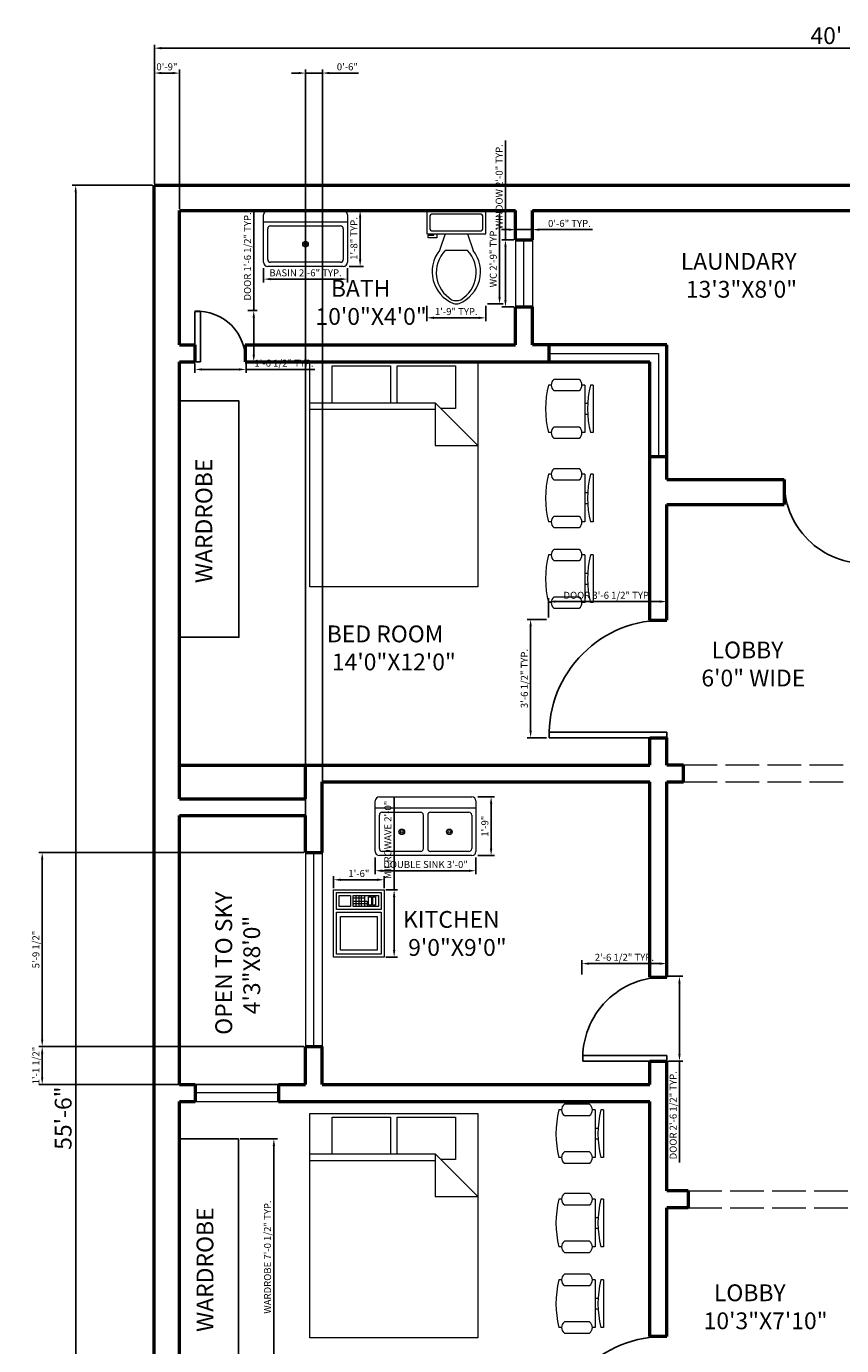
# Model space of a CAD drawing. Units: inches. Extents: x 2690 to 3266, y 1440 to 2261.
# Tile 3 of 4: x 2690 to 2981, y 1790 to 2261. Entities that reach past the tile are written whole.
import ezdxf

# ---------------------------------------------------------------- set-up
doc = ezdxf.new("R2010")
doc.units = ezdxf.units.IN
doc.linetypes.add('ACAD_ISO02W100', pattern=[15, 12, -3])
for name, color, linetype, lineweight in [('A-ANNO-DIMS', 2, 'Continuous', 18), ('A-ANNO-TEXT', 7, 'Continuous', 18), ('A-AREA-IDEN', 7, 'Continuous', 25), ('A-DOOR', 4, 'Continuous', 25), ('A-EQPM', 8, 'Continuous', 18), ('A-FLOR-CASE', 9, 'Continuous', 25), ('A-FLOR-FIXT', 9, 'Continuous', 18), ('A-FURN', 8, 'Continuous', 18), ('A-GLAZ', 3, 'Continuous', 18), ('A-WALL', 7, 'Continuous', 50), ('A-WALL-OVHD', 8, 'ACAD_ISO02W100', 18)]:
    doc.layers.add(name, color=color, linetype=linetype, lineweight=lineweight)
doc.styles.get("Standard").update_dxf_attribs({"font": 'arial.ttf'})
doc.dimstyles.new('ISO-25', dxfattribs={"dimtxt": 2.5, "dimasz": 2.5, "dimexe": 1.25, "dimexo": 0.625, "dimtad": 1, "dimlunit": 3, "dimtxsty": 'Standard', "dimcen": 2.5, "dimadec": 0, "dimazin": 0, "dimtfac": 1, "dimtmove": 0, "dimatfit": 3, "dimfxl": 1, "dimarcsym": 0})

# ---------------------------------------------------------------- blocks, each defined once
blk = doc.blocks.new('Sink-double - 36 in top')
for p, q in [((-18, -4), (18, -4)), ((-0.75, -18.5), (-0.75, -6.5)), ((0.75, -6.5), (0.75, -18.5))]:
    blk.add_line(p, q)
for points in [[(-16.5, 0), (16.5, 0)], [(-18, -19.5), (-18, -1.5)], [(18, -1.5), (18, -19.5)], [(-16.5, -18.5), (-16.5, -6.5)], [(-15.5, -5.5), (-1.75, -5.5)], [(1.75, -5.5), (15.5, -5.5)], [(16.5, -6.5), (16.5, -18.5)], [(16.5, -21), (-16.5, -21)], [(-1.75, -19.5), (-15.5, -19.5)], [(15.5, -19.5), (1.75, -19.5)]]:
    blk.add_lwpolyline(points)
for centre, radius in [((-8.5, -12.5), 1), ((-8.5, -12.5), 0.5), ((8.5, -12.5), 1), ((8.5, -12.5), 0.5)]:
    blk.add_circle(centre, radius)
for centre, radius, start, end in [((-16.5, -1.5), 1.5, 90, 180), ((16.5, -1.5), 1.5, 0, 90), ((-15.5, -6.5), 1, 90, 180), ((-1.75, -6.5), 1, 0, 90), ((1.75, -6.5), 1, 90, 180), ((15.5, -6.5), 1, 0, 90), ((-15.5, -18.5), 1, 180, 270), ((-1.75, -18.5), 1, 270, 0), ((1.75, -18.5), 1, 180, 270), ((15.5, -18.5), 1, 270, 0), ((-16.5, -19.5), 1.5, 180, 270), ((16.5, -19.5), 1.5, 270, 0)]:
    blk.add_arc(centre, radius, start, end)
blk = doc.blocks.new('Microwave')
for p, q in [((18, 10), (22, 10)), ((19, 7), (19, 11)), ((20, 11), (20, 7)), ((21, 7), (21, 11)), ((22, 9), (18, 9)), ((18, 8), (22, 8)), ((22, 7), (18, 7)), ((20, 6), (18, 6)), ((19, 6), (19, 7)), ((20, 7), (20, 6))]:
    blk.add_line(p, q)
for points in [[(0, 0), (0, 18), (24, 18), (24, 0)], [(1, 1), (1, 17), (16, 17), (16, 1)], [(2.5, 2.5), (2.5, 15.5), (14.5, 15.5), (14.5, 2.5)], [(17, 1), (17, 17), (23, 17), (23, 1)], [(18, 12), (18, 16), (22, 16), (22, 12)], [(18, 2), (18, 11), (22, 11), (22, 2)], [(18.5, 4.5), (18.5, 5.5), (21.5, 5.5), (21.5, 4.5)], [(18.5, 3), (18.5, 4), (21.5, 4), (21.5, 3)]]:
    blk.add_lwpolyline(points, close=True)
blk = doc.blocks.new('Toilet - top')
for p, q in [((9.5, -6), (9.5, -2)), ((-10, -8.5), (-8, -8.5)), ((-10, -9.5), (-10, -8.5)), ((-8, -8.5), (-8, -8)), ((-7, -8), (-7, -9.5)), ((-4, -8), (-6, -14)), ((4, -8), (6, -14)), ((-7, -9.5), (-10, -9.5)), ((4, -14), (-4, -14))]:
    blk.add_line(p, q)
blk.add_lwpolyline([(10.5, -8), (10.5, 0), (-10.5, 0), (-10.5, -8)], close=True)
for points in [[(-9.5, -2), (-9.5, -6)], [(8.5, -1), (-8.5, -1)], [(-8.5, -7), (8.5, -7)]]:
    blk.add_lwpolyline(points)
for centre, radius, start, end in [((-8.62, -1.88), 0.884, 81.8699, 188.1301), ((8.62, -1.88), 0.884, 351.8699, 98.1301), ((-8.62, -6.12), 0.884, 171.8699, 278.1301), ((8.62, -6.12), 0.884, 261.8699, 8.1301), ((3.52, -21.58), 12.17, 141.4691, 247.9714), ((4.2, -21.82), 11.33, 136.3677, 238.9468), ((-3.52, -21.58), 12.17, 292.0284, 38.5307), ((-4.2, -21.82), 11.33, 301.053, 43.6321), ((0, -27.88), 4, 245.7318, 294.2682), ((0, -29), 4, 254.8605, 285.1395)]:
    blk.add_arc(centre, radius, start, end)
blk = doc.blocks.new('Sink-single - 30 in top')
blk.add_line((-15, -3.999996), (15, -3.999996))
for points in [[(-13.5, 0), (13.5, 0)], [(-15, -18.499996), (-15, -1.5)], [(15, -1.5), (15, -18.499996)], [(-13.5, -17.499996), (-13.5, -6.499996)], [(-12.5, -5.499996), (12.5, -5.499996)], [(13.5, -6.499996), (13.5, -17.499996)], [(12.5, -18.499996), (-12.5, -18.499996)], [(13.5, -19.999996), (-13.5, -19.999996)]]:
    blk.add_lwpolyline(points)
for radius in [1, 0.5]:
    blk.add_circle((0, -11.999996), radius)
for centre, radius, start, end in [((-13.5, -1.5), 1.5, 90, 180), ((13.5, -1.5), 1.5, 0, 90), ((-12.5, -6.499996), 1, 90, 180), ((12.5, -6.499996), 1, 0, 90), ((-13.5, -18.499996), 1.5, 180, 270), ((-12.5, -17.499996), 1, 180, 270), ((12.5, -17.499996), 1, 270, 0), ((13.5, -18.499996), 1.5, 270, 0)]:
    blk.add_arc(centre, radius, start, end)
blk = doc.blocks.new('Bed - Queen')
for p, q in [((0, -80.00003), (0, 0)), ((0, 0), (59.99999, 0)), ((59.99999, 0), (59.99999, -80.00003)), ((7.99999, -1.2), (28.79998, -1.2)), ((7.99999, -14.4), (7.99999, -1.2)), ((28.79998, -1.2), (28.79998, -14.4)), ((31.19999, -1.2), (51.99999, -1.2)), ((31.19999, -14.4), (31.19999, -1.2)), ((51.99999, -1.2), (51.99999, -16.4)), ((0, -14.4), (44.8, -14.4)), ((44.8, -16.8), (0, -16.8)), ((59.99999, -29.6), (44.8, -14.4)), ((44.8, -14.4), (44.8, -29.6)), ((51.99999, -16.4), (46.79936, -16.4)), ((44.8, -29.6), (59.99999, -29.6)), ((59.99999, -80.00003), (0, -80.00003))]:
    blk.add_line(p, q)
blk = doc.blocks.new('Chair - Desk')
for p, q in [((-8.5, 0), (-8.5, -1)), ((-8.5, 0), (8.5, 0)), ((8.5, 0), (8.5, -1)), ((-8.5, -3), (-8.5, -4)), ((-8.5, -3), (8.5, -3)), ((-2, -3), (-2, -1.9355)), ((2, -1.9576), (2, -3)), ((8.5, -3), (8.5, -4)), ((-10.5, -5), (-10.5, -14)), ((-6.5, -14), (-6.5, -5)), ((6.5, -5), (6.5, -14)), ((10.5, -14), (10.5, -5)), ((-8.5, -15), (-8.5, -16)), ((8.5, -15), (8.5, -16))]:
    blk.add_line(p, q)
for centre, radius, start, end in [((-8.5, -6.5), 2.5, 36.8699, 143.1301), ((0, 34.625), 36.625, 256.5803, 283.4197), ((8.5, -6.5), 2.5, 36.8699, 143.1301), ((-8.5, -12.5), 2.5, 216.8699, 323.1301), ((8.5, -12.5), 2.5, 216.8699, 323.1301), ((0, 19.625), 36.625, 256.5803, 283.4197)]:
    blk.add_arc(centre, radius, start, end)
blk = doc.blocks.new('*D12')
at = {"layer": 'A-ANNO-DIMS', "color": 0, "lineweight": -2, "transparency": 16777216}
for p, q in [((2735.48, 2205.11), (2735.48, 2254.67)), ((2737.98, 2253.42), (3212.98, 2253.42)), ((3215.48, 2205.11), (3215.48, 2254.67))]:
    blk.add_line(p, q, dxfattribs=at)
at = {"layer": 'A-ANNO-DIMS', "color": 0, "transparency": 16777216}
for points in [[(2737.98, 2253.84), (2737.98, 2253.01), (2735.48, 2253.42)], [(3212.98, 2253.84), (3212.98, 2253.01), (3215.48, 2253.42)]]:
    blk.add_solid(points, dxfattribs=at)
at = {"layer": 'Defpoints', "color": 0, "transparency": 16777216}
for p in [(3215.48, 2253.42), (2735.48, 2204.49), (3215.48, 2204.49)]:
    blk.add_point(p, dxfattribs=at)
at = {"layer": 'A-ANNO-DIMS', "color": 0, "transparency": 16777216, "insert": (2975.48, 2257.11), "char_height": 6, "attachment_point": 5}
blk.add_mtext("40'", dxfattribs=at)
blk = doc.blocks.new('*D13')
at = {"layer": 'A-ANNO-DIMS', "color": 0, "lineweight": -2, "transparency": 16777216}
for p, q in [((2734.85, 2204.49), (2706.14, 2204.49)), ((2707.39, 1540.99), (2707.39, 2201.99)), ((2734.85, 1538.49), (2706.14, 1538.49))]:
    blk.add_line(p, q, dxfattribs=at)
at = {"layer": 'A-ANNO-DIMS', "color": 0, "transparency": 16777216}
for points in [[(2706.97, 2201.99), (2707.81, 2201.99), (2707.39, 2204.49)], [(2706.97, 1540.99), (2707.81, 1540.99), (2707.39, 1538.49)]]:
    blk.add_solid(points, dxfattribs=at)
at = {"layer": 'Defpoints', "color": 0, "transparency": 16777216}
for p in [(2707.39, 2204.49), (2735.48, 2204.49), (2735.48, 1538.49)]:
    blk.add_point(p, dxfattribs=at)
at = {"layer": 'A-ANNO-DIMS', "color": 0, "transparency": 16777216, "insert": (2703.7, 1871.49), "char_height": 6, "attachment_point": 5, "rotation": 90}
blk.add_mtext('55\'-6"', dxfattribs=at)
blk = doc.blocks.new('DOOR-SWING-18IN')
for p, q in [((0, 0), (0, 18)), ((0, 18), (2, 18)), ((2, 18), (2, 0)), ((2, 0), (0, 0))]:
    blk.add_line(p, q)
blk.add_arc((1, 1), 17.03, 356.6335, 93.3665)
blk = doc.blocks.new('DOOR-SWING-30IN')
for p, q in [((-2, -30), (-2, 0)), ((-2, 0), (0, 0)), ((0, 0), (0, -30)), ((0, -30), (-2, -30))]:
    blk.add_line(p, q)
blk.add_arc((-1, -1), 29.02, 178.0251, 271.9749)
blk = doc.blocks.new('DOOR-SWING-42IN')
for p, q in [((-42, 0), (-42, 2)), ((-42, 2), (0, 2)), ((0, 0), (-42, 0)), ((0, 2), (0, 0))]:
    blk.add_line(p, q)
blk.add_arc((-1, 1), 41.01, 88.6028, 181.3972)
blk = doc.blocks.new('WIN-24IN')
for p, q in [((0, 24), (0, 0)), ((3, 0), (3, 24)), ((3, 24), (6, 24)), ((6, 24), (6, 0)), ((0, 0), (3, 0))]:
    blk.add_line(p, q)
blk = doc.blocks.new('WARDROBE-PLAN')
blk.add_lwpolyline([(0, 0), (21.23, 0), (21.23, -84.36), (0, -84.36)], close=True)
blk = doc.blocks.new('*D23')
at = {"layer": 'A-ANNO-DIMS', "color": 0, "lineweight": -2, "transparency": 16777216}
for p, q in [((2876.2, 2050.17), (2876.2, 2057.13)), ((2878.7, 2055.88), (2915.98, 2055.88)), ((2918.48, 2050.17), (2918.48, 2057.13))]:
    blk.add_line(p, q, dxfattribs=at)
at = {"layer": 'A-ANNO-DIMS', "color": 0, "transparency": 16777216}
for points in [[(2878.7, 2056.3), (2878.7, 2055.47), (2876.2, 2055.88)], [(2915.98, 2056.3), (2915.98, 2055.47), (2918.48, 2055.88)]]:
    blk.add_solid(points, dxfattribs=at)
at = {"layer": 'Defpoints', "color": 0, "transparency": 16777216}
for p in [(2918.48, 2055.88), (2876.2, 2049.54), (2918.48, 2049.54)]:
    blk.add_point(p, dxfattribs=at)
at = {"layer": 'A-ANNO-DIMS', "color": 0, "transparency": 16777216, "insert": (2897.34, 2057.8), "char_height": 2.5, "attachment_point": 5}
blk.add_mtext('DOOR 3\'-6 1/2" TYP.', dxfattribs=at)
blk = doc.blocks.new('*D24')
at = {"layer": 'A-ANNO-DIMS', "color": 0, "lineweight": -2, "transparency": 16777216}
for p, q in [((2875.58, 2049.54), (2868.61, 2049.54)), ((2869.86, 2009.77), (2869.86, 2047.04)), ((2875.58, 2007.27), (2868.61, 2007.27))]:
    blk.add_line(p, q, dxfattribs=at)
at = {"layer": 'A-ANNO-DIMS', "color": 0, "transparency": 16777216}
for points in [[(2869.44, 2047.04), (2870.28, 2047.04), (2869.86, 2049.54)], [(2869.44, 2009.77), (2870.28, 2009.77), (2869.86, 2007.27)]]:
    blk.add_solid(points, dxfattribs=at)
at = {"layer": 'Defpoints', "color": 0, "transparency": 16777216}
for p in [(2869.86, 2049.54), (2876.2, 2049.54), (2876.2, 2007.27)]:
    blk.add_point(p, dxfattribs=at)
at = {"layer": 'A-ANNO-DIMS', "color": 0, "transparency": 16777216, "insert": (2867.94, 2028.41), "char_height": 2.5, "attachment_point": 5, "rotation": 90}
blk.add_mtext('3\'-6 1/2" TYP.', dxfattribs=at)
blk = doc.blocks.new('*D25')
at = {"layer": 'A-ANNO-DIMS', "color": 0, "lineweight": -2, "transparency": 16777216}
for p, q in [((2854.43, 2195.18), (2860.02, 2195.18)), ((2858.77, 2164.63), (2858.77, 2192.68)), ((2854.43, 2162.13), (2860.02, 2162.13))]:
    blk.add_line(p, q, dxfattribs=at)
at = {"layer": 'A-ANNO-DIMS', "color": 0, "transparency": 16777216}
for points in [[(2858.35, 2192.68), (2859.18, 2192.68), (2858.77, 2195.18)], [(2858.35, 2164.63), (2859.18, 2164.63), (2858.77, 2162.13)]]:
    blk.add_solid(points, dxfattribs=at)
at = {"layer": 'Defpoints', "color": 0, "transparency": 16777216}
for p in [(2853.81, 2195.18), (2858.77, 2195.18), (2853.81, 2162.13)]:
    blk.add_point(p, dxfattribs=at)
at = {"layer": 'A-ANNO-DIMS', "color": 0, "transparency": 16777216, "insert": (2856.85, 2178.65), "char_height": 2.5, "attachment_point": 5, "rotation": 90}
blk.add_mtext('WC 2\'-9" TYP.', dxfattribs=at)
blk = doc.blocks.new('*D26')
at = {"layer": 'A-ANNO-DIMS', "color": 0, "lineweight": -2, "transparency": 16777216}
for p, q in [((2832.81, 2161.5), (2832.81, 2155.92)), ((2853.81, 2161.5), (2853.81, 2155.92)), ((2835.31, 2157.17), (2851.31, 2157.17))]:
    blk.add_line(p, q, dxfattribs=at)
at = {"layer": 'A-ANNO-DIMS', "color": 0, "transparency": 16777216}
for points in [[(2835.31, 2157.59), (2835.31, 2156.76), (2832.81, 2157.17)], [(2851.31, 2157.59), (2851.31, 2156.76), (2853.81, 2157.17)]]:
    blk.add_solid(points, dxfattribs=at)
at = {"layer": 'Defpoints', "color": 0, "transparency": 16777216}
for p in [(2832.81, 2162.13), (2853.81, 2162.13), (2853.81, 2157.17)]:
    blk.add_point(p, dxfattribs=at)
at = {"layer": 'A-ANNO-DIMS', "color": 0, "transparency": 16777216, "insert": (2843.31, 2159.07), "char_height": 2.5, "attachment_point": 5}
blk.add_mtext('1\'-9" TYP.', dxfattribs=at)
blk = doc.blocks.new('*D27')
at = {"layer": 'A-ANNO-DIMS', "color": 0, "lineweight": -2, "transparency": 16777216}
for p, q in [((2774.48, 2174.86), (2774.48, 2169.74)), ((2776.98, 2170.99), (2801.98, 2170.99)), ((2804.48, 2174.86), (2804.48, 2169.74))]:
    blk.add_line(p, q, dxfattribs=at)
at = {"layer": 'A-ANNO-DIMS', "color": 0, "transparency": 16777216}
for points in [[(2776.98, 2171.4), (2776.98, 2170.57), (2774.48, 2170.99)], [(2801.98, 2171.4), (2801.98, 2170.57), (2804.48, 2170.99)]]:
    blk.add_solid(points, dxfattribs=at)
at = {"layer": 'Defpoints', "color": 0, "transparency": 16777216}
for p in [(2774.48, 2175.49), (2804.48, 2175.49), (2804.48, 2170.99)]:
    blk.add_point(p, dxfattribs=at)
at = {"layer": 'A-ANNO-DIMS', "color": 0, "transparency": 16777216, "insert": (2789.48, 2172.9), "char_height": 2.5, "attachment_point": 5}
blk.add_mtext('BASIN 2\'-6" TYP.', dxfattribs=at)
blk = doc.blocks.new('*D28')
at = {"layer": 'A-ANNO-DIMS', "color": 0, "lineweight": -2, "transparency": 16777216}
for p, q in [((2805.1, 2195.49), (2810.23, 2195.49)), ((2808.98, 2177.99), (2808.98, 2192.99)), ((2805.1, 2175.49), (2810.23, 2175.49))]:
    blk.add_line(p, q, dxfattribs=at)
at = {"layer": 'A-ANNO-DIMS', "color": 0, "transparency": 16777216}
for points in [[(2808.56, 2192.99), (2809.39, 2192.99), (2808.98, 2195.49)], [(2808.56, 2177.99), (2809.39, 2177.99), (2808.98, 2175.49)]]:
    blk.add_solid(points, dxfattribs=at)
at = {"layer": 'Defpoints', "color": 0, "transparency": 16777216}
for p in [(2804.48, 2195.49), (2808.98, 2195.49), (2804.48, 2175.49)]:
    blk.add_point(p, dxfattribs=at)
at = {"layer": 'A-ANNO-DIMS', "color": 0, "transparency": 16777216, "insert": (2807.07, 2185.49), "char_height": 2.5, "attachment_point": 5, "rotation": 90}
blk.add_mtext('1\'-8" TYP.', dxfattribs=at)
blk = doc.blocks.new('*D31')
at = {"layer": 'A-ANNO-DIMS', "color": 0, "lineweight": -2, "transparency": 16777216}
for p, q in [((2766.13, 1864.09), (2779.41, 1864.09)), ((2778.16, 1782.23), (2778.16, 1861.59)), ((2766.13, 1779.73), (2779.41, 1779.73))]:
    blk.add_line(p, q, dxfattribs=at)
at = {"layer": 'A-ANNO-DIMS', "color": 0, "transparency": 16777216}
for points in [[(2777.74, 1861.59), (2778.58, 1861.59), (2778.16, 1864.09)], [(2777.74, 1782.23), (2778.58, 1782.23), (2778.16, 1779.73)]]:
    blk.add_solid(points, dxfattribs=at)
at = {"layer": 'Defpoints', "color": 0, "transparency": 16777216}
for p in [(2765.51, 1864.09), (2778.16, 1864.09), (2765.51, 1779.73)]:
    blk.add_point(p, dxfattribs=at)
at = {"layer": 'A-ANNO-DIMS', "color": 0, "transparency": 16777216, "insert": (2776.24, 1821.91), "char_height": 2.5, "attachment_point": 5, "rotation": 90}
blk.add_mtext('WARDROBE 7\'-0 1/2" TYP.', dxfattribs=at)
blk = doc.blocks.new('*D35')
at = {"layer": 'A-ANNO-DIMS', "color": 0, "lineweight": -2, "transparency": 16777216}
for p, q in [((2770.99, 2159.77), (2770.99, 2195.91)), ((2768.87, 2159.77), (2772.24, 2159.77)), ((2770.99, 2143.99), (2770.99, 2157.27)), ((2768.87, 2141.49), (2772.24, 2141.49))]:
    blk.add_line(p, q, dxfattribs=at)
at = {"layer": 'A-ANNO-DIMS', "color": 0, "transparency": 16777216}
for points in [[(2770.57, 2157.27), (2771.4, 2157.27), (2770.99, 2159.77)], [(2770.57, 2143.99), (2771.4, 2143.99), (2770.99, 2141.49)]]:
    blk.add_solid(points, dxfattribs=at)
at = {"layer": 'Defpoints', "color": 0, "transparency": 16777216}
for p in [(2768.24, 2159.77), (2770.99, 2159.77), (2768.24, 2141.49)]:
    blk.add_point(p, dxfattribs=at)
at = {"layer": 'A-ANNO-DIMS', "color": 0, "transparency": 16777216, "insert": (2769.07, 2179.09), "char_height": 2.5, "attachment_point": 5, "rotation": 90}
blk.add_mtext('DOOR 1\'-6 1/2" TYP.', dxfattribs=at)
blk = doc.blocks.new('*D36')
at = {"layer": 'A-ANNO-DIMS', "color": 0, "lineweight": -2, "transparency": 16777216}
for p, q in [((2749.96, 2140.86), (2749.96, 2137.49)), ((2752.46, 2138.74), (2765.74, 2138.74)), ((2768.24, 2140.86), (2768.24, 2137.49)), ((2768.24, 2138.74), (2792.82, 2138.74))]:
    blk.add_line(p, q, dxfattribs=at)
at = {"layer": 'A-ANNO-DIMS', "color": 0, "transparency": 16777216}
for points in [[(2752.46, 2139.16), (2752.46, 2138.33), (2749.96, 2138.74)], [(2765.74, 2139.16), (2765.74, 2138.33), (2768.24, 2138.74)]]:
    blk.add_solid(points, dxfattribs=at)
at = {"layer": 'Defpoints', "color": 0, "transparency": 16777216}
for p in [(2749.96, 2141.49), (2768.24, 2141.49), (2768.24, 2138.74)]:
    blk.add_point(p, dxfattribs=at)
at = {"layer": 'A-ANNO-DIMS', "color": 0, "transparency": 16777216, "insert": (2781.78, 2140.66), "char_height": 2.5, "attachment_point": 5}
blk.add_mtext('1\'-6 1/2" TYP.', dxfattribs=at)
blk = doc.blocks.new('*D37')
at = {"layer": 'A-ANNO-DIMS', "color": 0, "lineweight": -2, "transparency": 16777216}
for p, q in [((2919.1, 1922.11), (2924.27, 1922.11)), ((2923.02, 1919.61), (2923.02, 1894.34)), ((2919.1, 1891.84), (2924.27, 1891.84)), ((2923.02, 1891.84), (2923.02, 1855.7))]:
    blk.add_line(p, q, dxfattribs=at)
at = {"layer": 'A-ANNO-DIMS', "color": 0, "transparency": 16777216}
for points in [[(2922.6, 1919.61), (2923.43, 1919.61), (2923.02, 1922.11)], [(2922.6, 1894.34), (2923.43, 1894.34), (2923.02, 1891.84)]]:
    blk.add_solid(points, dxfattribs=at)
at = {"layer": 'Defpoints', "color": 0, "transparency": 16777216}
for p in [(2918.48, 1922.11), (2918.48, 1891.84), (2923.02, 1891.84)]:
    blk.add_point(p, dxfattribs=at)
at = {"layer": 'A-ANNO-DIMS', "color": 0, "transparency": 16777216, "insert": (2921.1, 1872.52), "char_height": 2.5, "attachment_point": 5, "rotation": 90}
blk.add_mtext('DOOR 2\'-6 1/2" TYP.', dxfattribs=at)
blk = doc.blocks.new('*D38')
at = {"layer": 'A-ANNO-DIMS', "color": 0, "lineweight": -2, "transparency": 16777216}
for p, q in [((2888.2, 1922.74), (2888.2, 1927.9)), ((2890.7, 1926.65), (2915.98, 1926.65)), ((2918.48, 1922.74), (2918.48, 1927.9))]:
    blk.add_line(p, q, dxfattribs=at)
at = {"layer": 'A-ANNO-DIMS', "color": 0, "transparency": 16777216}
for points in [[(2890.7, 1927.07), (2890.7, 1926.24), (2888.2, 1926.65)], [(2915.98, 1927.07), (2915.98, 1926.24), (2918.48, 1926.65)]]:
    blk.add_solid(points, dxfattribs=at)
at = {"layer": 'Defpoints', "color": 0, "transparency": 16777216}
for p in [(2918.48, 1926.65), (2888.2, 1922.11), (2918.48, 1922.11)]:
    blk.add_point(p, dxfattribs=at)
at = {"layer": 'A-ANNO-DIMS', "color": 0, "transparency": 16777216, "insert": (2903.34, 1928.57), "char_height": 2.5, "attachment_point": 5}
blk.add_mtext('2\'-6 1/2" TYP.', dxfattribs=at)
blk = doc.blocks.new('*D39')
at = {"layer": 'A-ANNO-DIMS', "color": 0, "lineweight": -2, "transparency": 16777216}
for p, q in [((2860.88, 2185.04), (2860.88, 2220.43)), ((2863.85, 2185.04), (2859.63, 2185.04)), ((2860.88, 2163.54), (2860.88, 2182.54)), ((2863.85, 2161.04), (2859.63, 2161.04))]:
    blk.add_line(p, q, dxfattribs=at)
at = {"layer": 'A-ANNO-DIMS', "color": 0, "transparency": 16777216}
for points in [[(2860.46, 2182.54), (2861.29, 2182.54), (2860.88, 2185.04)], [(2860.46, 2163.54), (2861.29, 2163.54), (2860.88, 2161.04)]]:
    blk.add_solid(points, dxfattribs=at)
at = {"layer": 'Defpoints', "color": 0, "transparency": 16777216}
for p in [(2860.88, 2185.04), (2864.48, 2185.04), (2864.48, 2161.04)]:
    blk.add_point(p, dxfattribs=at)
at = {"layer": 'A-ANNO-DIMS', "color": 0, "transparency": 16777216, "insert": (2858.96, 2203.98), "char_height": 2.5, "attachment_point": 5, "rotation": 90}
blk.add_mtext('WINDOW 2\'-0" TYP.', dxfattribs=at)
blk = doc.blocks.new('*D40')
at = {"layer": 'A-ANNO-DIMS', "color": 0, "lineweight": -2, "transparency": 16777216}
for p, q in [((2864.48, 2185.67), (2864.48, 2189.89)), ((2870.48, 2185.67), (2870.48, 2189.89)), ((2861.98, 2188.64), (2859.48, 2188.64)), ((2864.48, 2188.64), (2870.48, 2188.64)), ((2872.98, 2188.64), (2891.97, 2188.64))]:
    blk.add_line(p, q, dxfattribs=at)
at = {"layer": 'A-ANNO-DIMS', "color": 0, "transparency": 16777216}
for points in [[(2861.98, 2189.06), (2861.98, 2188.22), (2864.48, 2188.64)], [(2872.98, 2189.06), (2872.98, 2188.22), (2870.48, 2188.64)]]:
    blk.add_solid(points, dxfattribs=at)
at = {"layer": 'Defpoints', "color": 0, "transparency": 16777216}
for p in [(2864.48, 2185.04), (2870.48, 2188.64), (2870.48, 2185.04)]:
    blk.add_point(p, dxfattribs=at)
at = {"layer": 'A-ANNO-DIMS', "color": 0, "transparency": 16777216, "insert": (2883.72, 2190.54), "char_height": 2.5, "attachment_point": 5}
blk.add_mtext('0\'-6" TYP.', dxfattribs=at)
blk = doc.blocks.new('*D43')
at = {"layer": 'A-ANNO-DIMS', "color": 0, "lineweight": -2, "transparency": 16777216}
for p, q in [((2814.35, 1964.57), (2814.35, 1958.55)), ((2850.35, 1964.57), (2850.35, 1958.55)), ((2816.85, 1959.8), (2847.85, 1959.8))]:
    blk.add_line(p, q, dxfattribs=at)
at = {"layer": 'A-ANNO-DIMS', "color": 0, "transparency": 16777216}
for points in [[(2816.85, 1960.21), (2816.85, 1959.38), (2814.35, 1959.8)], [(2847.85, 1960.21), (2847.85, 1959.38), (2850.35, 1959.8)]]:
    blk.add_solid(points, dxfattribs=at)
at = {"layer": 'Defpoints', "color": 0, "transparency": 16777216}
for p in [(2814.35, 1965.2), (2850.35, 1965.2), (2850.35, 1959.8)]:
    blk.add_point(p, dxfattribs=at)
at = {"layer": 'A-ANNO-DIMS', "color": 0, "transparency": 16777216, "insert": (2832.35, 1961.72), "char_height": 2.5, "attachment_point": 5}
blk.add_mtext('DOUBLE SINK 3\'-0"', dxfattribs=at)
blk = doc.blocks.new('*D44')
at = {"layer": 'A-ANNO-DIMS', "color": 0, "lineweight": -2, "transparency": 16777216}
for p, q in [((2850.97, 1986.2), (2857, 1986.2)), ((2855.75, 1967.7), (2855.75, 1983.7)), ((2850.97, 1965.2), (2857, 1965.2))]:
    blk.add_line(p, q, dxfattribs=at)
at = {"layer": 'A-ANNO-DIMS', "color": 0, "transparency": 16777216}
for points in [[(2855.33, 1983.7), (2856.17, 1983.7), (2855.75, 1986.2)], [(2855.33, 1967.7), (2856.17, 1967.7), (2855.75, 1965.2)]]:
    blk.add_solid(points, dxfattribs=at)
at = {"layer": 'Defpoints', "color": 0, "transparency": 16777216}
for p in [(2850.35, 1986.2), (2855.75, 1986.2), (2850.35, 1965.2)]:
    blk.add_point(p, dxfattribs=at)
at = {"layer": 'A-ANNO-DIMS', "color": 0, "transparency": 16777216, "insert": (2853.85, 1975.7), "char_height": 2.5, "attachment_point": 5, "rotation": 90}
blk.add_mtext('1\'-9"', dxfattribs=at)
blk = doc.blocks.new('*D45')
at = {"layer": 'A-ANNO-DIMS', "color": 0, "lineweight": -2, "transparency": 16777216}
for p, q in [((2821.12, 1952.98), (2821.12, 1986.16)), ((2818.14, 1952.98), (2822.37, 1952.98)), ((2821.12, 1931.48), (2821.12, 1950.48)), ((2818.14, 1928.98), (2822.37, 1928.98))]:
    blk.add_line(p, q, dxfattribs=at)
at = {"layer": 'A-ANNO-DIMS', "color": 0, "transparency": 16777216}
for points in [[(2820.7, 1950.48), (2821.54, 1950.48), (2821.12, 1952.98)], [(2820.7, 1931.48), (2821.54, 1931.48), (2821.12, 1928.98)]]:
    blk.add_solid(points, dxfattribs=at)
at = {"layer": 'Defpoints', "color": 0, "transparency": 16777216}
for p in [(2817.52, 1952.98), (2821.12, 1952.98), (2817.52, 1928.98)]:
    blk.add_point(p, dxfattribs=at)
at = {"layer": 'A-ANNO-DIMS', "color": 0, "transparency": 16777216, "insert": (2819.2, 1970.82), "char_height": 2.5, "attachment_point": 5, "rotation": 90}
blk.add_mtext('MICROWAVE 2\'-0"', dxfattribs=at)
blk = doc.blocks.new('*D46')
at = {"layer": 'A-ANNO-DIMS', "color": 0, "lineweight": -2, "transparency": 16777216}
for p, q in [((2799.52, 1953.61), (2799.52, 1957.83)), ((2815.02, 1956.58), (2802.02, 1956.58)), ((2817.52, 1953.61), (2817.52, 1957.83))]:
    blk.add_line(p, q, dxfattribs=at)
at = {"layer": 'A-ANNO-DIMS', "color": 0, "transparency": 16777216}
for points in [[(2802.02, 1957), (2802.02, 1956.16), (2799.52, 1956.58)], [(2815.02, 1957), (2815.02, 1956.16), (2817.52, 1956.58)]]:
    blk.add_solid(points, dxfattribs=at)
at = {"layer": 'Defpoints', "color": 0, "transparency": 16777216}
for p in [(2799.52, 1956.58), (2799.52, 1952.98), (2817.52, 1952.98)]:
    blk.add_point(p, dxfattribs=at)
at = {"layer": 'A-ANNO-DIMS', "color": 0, "transparency": 16777216, "insert": (2808.52, 1958.48), "char_height": 2.5, "attachment_point": 5}
blk.add_mtext('1\'-6"', dxfattribs=at)
blk = doc.blocks.new('*D54')
at = {"layer": 'A-ANNO-DIMS', "color": 0, "lineweight": -2, "transparency": 16777216}
for p, q in [((2735.48, 2205.11), (2735.48, 2245.79)), ((2737.98, 2244.54), (2741.98, 2244.54)), ((2744.48, 2196.11), (2744.48, 2245.79))]:
    blk.add_line(p, q, dxfattribs=at)
at = {"layer": 'A-ANNO-DIMS', "color": 0, "transparency": 16777216}
for points in [[(2737.98, 2244.95), (2737.98, 2244.12), (2735.48, 2244.54)], [(2741.98, 2244.95), (2741.98, 2244.12), (2744.48, 2244.54)]]:
    blk.add_solid(points, dxfattribs=at)
at = {"layer": 'Defpoints', "color": 0, "transparency": 16777216}
for p in [(2744.48, 2244.54), (2735.48, 2204.49), (2744.48, 2195.49)]:
    blk.add_point(p, dxfattribs=at)
at = {"layer": 'A-ANNO-DIMS', "color": 0, "transparency": 16777216, "insert": (2739.98, 2246.44), "char_height": 2.5, "attachment_point": 5}
blk.add_mtext('0\'-9"', dxfattribs=at)
blk = doc.blocks.new('*D55')
at = {"layer": 'A-ANNO-DIMS', "color": 0, "lineweight": -2, "transparency": 16777216}
for p, q in [((2786.98, 2244.54), (2784.48, 2244.54)), ((2789.48, 1966.94), (2789.48, 2245.79)), ((2789.48, 2244.54), (2795.48, 2244.54)), ((2795.48, 1966.94), (2795.48, 2245.79)), ((2797.98, 2244.54), (2808.37, 2244.54))]:
    blk.add_line(p, q, dxfattribs=at)
at = {"layer": 'A-ANNO-DIMS', "color": 0, "transparency": 16777216}
for points in [[(2786.98, 2244.95), (2786.98, 2244.12), (2789.48, 2244.54)], [(2797.98, 2244.95), (2797.98, 2244.12), (2795.48, 2244.54)]]:
    blk.add_solid(points, dxfattribs=at)
at = {"layer": 'Defpoints', "color": 0, "transparency": 16777216}
for p in [(2795.48, 2244.54), (2789.48, 1966.32), (2795.48, 1966.32)]:
    blk.add_point(p, dxfattribs=at)
at = {"layer": 'A-ANNO-DIMS', "color": 0, "transparency": 16777216, "insert": (2804.42, 2246.44), "char_height": 2.5, "attachment_point": 5}
blk.add_mtext('0\'-6"', dxfattribs=at)
blk = doc.blocks.new('*D56')
at = {"layer": 'A-ANNO-DIMS', "color": 0, "lineweight": -2, "transparency": 16777216}
for p, q in [((2788.85, 1966.32), (2694.18, 1966.32)), ((2695.43, 1899.54), (2695.43, 1963.82)), ((2788.85, 1897.04), (2694.18, 1897.04))]:
    blk.add_line(p, q, dxfattribs=at)
at = {"layer": 'A-ANNO-DIMS', "color": 0, "transparency": 16777216}
for points in [[(2695.01, 1963.82), (2695.84, 1963.82), (2695.43, 1966.32)], [(2695.01, 1899.54), (2695.84, 1899.54), (2695.43, 1897.04)]]:
    blk.add_solid(points, dxfattribs=at)
at = {"layer": 'Defpoints', "color": 0, "transparency": 16777216}
for p in [(2695.43, 1966.32), (2789.48, 1966.32), (2789.48, 1897.04)]:
    blk.add_point(p, dxfattribs=at)
at = {"layer": 'A-ANNO-DIMS', "color": 0, "transparency": 16777216, "insert": (2693.51, 1931.68), "char_height": 2.5, "attachment_point": 5, "rotation": 90}
blk.add_mtext('5\'-9 1/2"', dxfattribs=at)
blk = doc.blocks.new('*D57')
at = {"layer": 'A-ANNO-DIMS', "color": 0, "lineweight": -2, "transparency": 16777216}
for p, q in [((2788.85, 1897.04), (2694.18, 1897.04)), ((2695.43, 1885.99), (2695.43, 1894.54)), ((2788.85, 1883.49), (2694.18, 1883.49))]:
    blk.add_line(p, q, dxfattribs=at)
at = {"layer": 'A-ANNO-DIMS', "color": 0, "transparency": 16777216}
for points in [[(2695.01, 1894.54), (2695.84, 1894.54), (2695.43, 1897.04)], [(2695.01, 1885.99), (2695.84, 1885.99), (2695.43, 1883.49)]]:
    blk.add_solid(points, dxfattribs=at)
at = {"layer": 'Defpoints', "color": 0, "transparency": 16777216}
for p in [(2695.43, 1897.04), (2789.48, 1897.04), (2789.48, 1883.49)]:
    blk.add_point(p, dxfattribs=at)
at = {"layer": 'A-ANNO-DIMS', "color": 0, "transparency": 16777216, "insert": (2693.51, 1890.26), "char_height": 2.5, "attachment_point": 5, "rotation": 90}
blk.add_mtext('1\'-1 1/2"', dxfattribs=at)

msp = doc.modelspace()

# ---------------------------------------------------------------- linework, layer by layer
at = {"layer": 'A-GLAZ'}
for p, q in [((2876.476, 2144.486), (2915.476, 2144.486)), ((2915.476, 2144.486), (2915.476, 2107.646)), ((2789.476, 1966.319), (2789.476, 1897.042)), ((2792.476, 1897.042), (2792.476, 1966.319)), ((2792.476, 1966.319), (2795.476, 1966.319)), ((2795.476, 1966.319), (2795.476, 1897.042)), ((2789.476, 1897.042), (2792.476, 1897.042)), ((2750.119, 1880.486), (2750.119, 1883.486)), ((2750.119, 1883.486), (2779.77, 1883.486)), ((2779.77, 1880.486), (2750.119, 1880.486)), ((2779.77, 1877.486), (2779.77, 1880.486)), ((2750.119, 1877.486), (2779.77, 1877.486))]:
    msp.add_line(p, q, dxfattribs=at)
at = {"layer": 'A-WALL'}
for p, q in [((2735.476, 2204.486), (3215.476, 2204.486)), ((2735.476, 1538.486), (2735.476, 2204.486)), ((2744.476, 2195.486), (2864.476, 2195.486)), ((2744.476, 2147.486), (2744.476, 2195.486)), ((2864.476, 2185.041), (2864.476, 2195.486)), ((2870.476, 2195.486), (3026.476, 2195.486)), ((2870.476, 2185.041), (2870.476, 2195.486)), ((2864.476, 2185.041), (2870.476, 2185.041)), ((2864.476, 2147.486), (2864.476, 2161.041)), ((2864.476, 2161.041), (2870.476, 2161.041)), ((2870.476, 2147.486), (2870.476, 2161.041)), ((2744.476, 2147.486), (2749.959, 2147.486)), ((2749.959, 2147.486), (2749.959, 2141.486)), ((2767.959, 2147.486), (2767.959, 2141.486)), ((2767.959, 2147.486), (2864.476, 2147.486)), ((2876.476, 2147.486), (2870.476, 2147.486)), ((2876.476, 2141.486), (2876.476, 2147.486)), ((2918.476, 2147.486), (2876.476, 2147.486)), ((2918.476, 2141.486), (2918.476, 2147.486)), ((2744.476, 2141.486), (2749.959, 2141.486)), ((2744.476, 1985.486), (2744.476, 2141.486)), ((2767.959, 2141.486), (2870.476, 2141.486)), ((2870.476, 2141.486), (2876.476, 2141.486)), ((2876.476, 2141.486), (2912.476, 2141.486)), ((2912.476, 2049.268), (2912.476, 2141.486)), ((2918.476, 2099.486), (2918.476, 2141.486)), ((2912.476, 2107.646), (2918.476, 2107.646)), ((2918.476, 2099.486), (2960.461, 2099.486)), ((2960.461, 2099.486), (2960.461, 2090.486)), ((2918.476, 2090.486), (2960.461, 2090.486)), ((2918.476, 2049.268), (2918.476, 2090.486)), ((2912.476, 2049.268), (2918.476, 2049.268)), ((2912.476, 2007.268), (2918.476, 2007.268)), ((2912.476, 1997.486), (2912.476, 2007.268)), ((2918.476, 1997.486), (2918.476, 2007.268)), ((2744.476, 1997.486), (2912.476, 1997.486)), ((2789.476, 1985.486), (2789.476, 1997.486)), ((2924.476, 1997.486), (2918.476, 1997.486)), ((2924.476, 1991.486), (2924.476, 1997.486)), ((2795.476, 1991.486), (2912.476, 1991.486)), ((2795.476, 1966.319), (2795.476, 1991.486)), ((2912.476, 1921.836), (2912.476, 1991.486)), ((2918.476, 1991.486), (2924.476, 1991.486)), ((2918.476, 1921.836), (2918.476, 1991.486)), ((2744.476, 1985.486), (2789.476, 1985.486)), ((2744.476, 1979.486), (2789.476, 1979.486)), ((2744.476, 1883.486), (2744.476, 1979.486)), ((2789.476, 1966.319), (2789.476, 1979.486)), ((2789.476, 1966.319), (2795.476, 1966.319)), ((2912.476, 1921.836), (2918.476, 1921.836)), ((2789.476, 1883.486), (2789.476, 1897.042)), ((2789.476, 1897.042), (2795.476, 1897.042)), ((2795.476, 1883.486), (2795.476, 1897.042)), ((2912.476, 1891.836), (2918.476, 1891.836)), ((2912.476, 1883.486), (2912.476, 1891.836)), ((2918.476, 1845.486), (2918.476, 1891.836)), ((2744.476, 1883.486), (2750.119, 1883.486)), ((2750.119, 1883.486), (2750.119, 1877.486)), ((2779.77, 1883.486), (2779.77, 1877.486)), ((2779.77, 1883.486), (2789.476, 1883.486)), ((2795.476, 1883.486), (2912.476, 1883.486)), ((2744.476, 1877.486), (2750.119, 1877.486)), ((2744.476, 1745.486), (2744.476, 1877.486)), ((2779.77, 1877.486), (2912.476, 1877.486)), ((2912.476, 1793.486), (2912.476, 1877.486)), ((2926.112, 1845.486), (2918.476, 1845.486)), ((2926.112, 1845.486), (2926.112, 1839.486)), ((2918.476, 1793.486), (2918.476, 1839.486)), ((2926.112, 1839.486), (2918.476, 1839.486)), ((2918.476, 1793.486), (2912.476, 1793.486))]:
    msp.add_line(p, q, dxfattribs=at)
at = {"layer": 'A-WALL-OVHD'}
for p, q in [((2996.476, 1997.486), (2924.476, 1997.486)), ((2924.476, 1991.486), (2996.476, 1991.486)), ((2926.112, 1845.486), (3041.476, 1845.486)), ((2926.112, 1839.486), (3041.476, 1839.486))]:
    msp.add_line(p, q, dxfattribs=at)

# ---------------------------------------------------------------- block references
at = {"layer": 'A-DOOR'}
for name, p in [('DOOR-SWING-18IN', (2749.959, 2141.486)), ('DOOR-SWING-30IN', (2990.461, 2099.486)), ('DOOR-SWING-42IN', (2918.476, 2007.268)), ('DOOR-SWING-42IN', (2918.476, 1751.486))]:
    msp.add_blockref(name, p, dxfattribs=at)
at = {"layer": 'A-DOOR', "rotation": 270.0000000000015}
msp.add_blockref('DOOR-SWING-30IN', (2918.476, 1891.836), dxfattribs=at)
at = {"layer": 'A-EQPM', "rotation": 90}
msp.add_blockref('Microwave', (2817.52, 1928.98), dxfattribs=at)
at = {"layer": 'A-FLOR-CASE'}
for p in [(2744.475, 2127.504), (2744.283, 1864.093)]:
    msp.add_blockref('WARDROBE-PLAN', p, dxfattribs=at)
at = {"layer": 'A-FLOR-FIXT'}
for name, p in [('Sink-single - 30 in top', (2789.476, 2195.486)), ('Toilet - top', (2843.309, 2195.175)), ('Sink-double - 36 in top', (2832.35, 1986.197))]:
    msp.add_blockref(name, p, dxfattribs=at)
at = {"layer": 'A-FURN'}
for p in [(2791.031, 2141.193), (2791.031, 1873.095)]:
    msp.add_blockref('Bed - Queen', p, dxfattribs=at)
at = {"layer": 'A-FURN', "rotation": 270}
for p in [(2892.21, 2124.681), (2892.21, 2092.803), (2892.21, 2064.01), (2895.916, 1865.926), (2895.916, 1834.048), (2895.916, 1805.255)]:
    msp.add_blockref('Chair - Desk', p, dxfattribs=at)
at = {"layer": 'A-GLAZ'}
msp.add_blockref('WIN-24IN', (2864.476, 2161.041), dxfattribs=at)

# ---------------------------------------------------------------- texts
at = {"layer": 'A-ANNO-TEXT', "char_height": 6, "attachment_point": 1, "rotation": 90}
for insert in [(2750.16, 2056.961), (2750.564, 1789.672)]:
    msp.add_mtext_dynamic_manual_height_columns('   WARDROBE', width=77.52183, gutter_width=12.5, heights=[0], dxfattribs=dict(at, insert=insert))
at = {"layer": 'A-AREA-IDEN', "char_height": 6, "attachment_point": 1}
for s, insert in [('    LAUNDARY\\P     13\'3"X8\'0"', (2916.147, 2180.354)), ('    BATH\\P 10\'0"X4\'0"', (2791.194, 2170.665)), ('      BED ROOM\\P       14\'0"X12\'0"', (2786.055, 2047.344)), ('      LOBBY\\P    6\'0" WIDE', (2923.507, 2041.588)), (' KITCHEN\\P  9\'0"X9\'0"', (2822.466, 1945.424)), ('  LOBBY\\P10\'3"X7\'10"', (2931.651, 1812.143))]:
    msp.add_mtext_dynamic_manual_height_columns(s, width=77.52183, gutter_width=12.5, heights=[0], dxfattribs=dict(at, insert=insert))
at = {"layer": 'A-AREA-IDEN', "insert": (2757.267, 1895.728), "char_height": 6, "attachment_point": 1, "rotation": 90}
msp.add_mtext_dynamic_manual_height_columns('   OPEN TO SKY\\P       4\'3"X8\'0"', width=77.52183, gutter_width=12.5, heights=[0], dxfattribs=at)

# ---------------------------------------------------------------- dimensions: what is measured, and where the dimension line sits
at = {"layer": 'A-ANNO-DIMS'}
for base, p1, p2, override, picture, middle in [((3215.476, 2253.424), (2735.476, 2204.486), (3215.476, 2204.486), {"dimtxt": 6, "dimclrd": 0, "dimclre": 0, "dimclrt": 0}, '*D12', (2975.476, 2257.113)), ((2744.476, 2244.536), (2735.476, 2204.486), (2744.476, 2195.486), {"dimdec": 1, "dimlfac": 1, "dimrnd": 0, "dimzin": 1, "dimdsep": 46, "dimlunit": 4, "dimfrac": 2}, '*D54', (2739.976, 2246.437)), ((2795.476, 2244.536), (2789.476, 1966.319), (2795.476, 1966.319), {"dimdec": 1, "dimlfac": 1, "dimrnd": 0, "dimzin": 1, "dimdsep": 46, "dimlunit": 4, "dimfrac": 2}, '*D55', (2804.424, 2246.437))]:
    dim = msp.add_linear_dim(base=base, p1=p1, p2=p2, dimstyle='ISO-25', override=override, dxfattribs=at)
    dim.commit()
    dim.dimension.update_dxf_attribs({"geometry": picture, "text_midpoint": middle})
for base, p1, p2, angle, text, picture, middle in [((2860.876, 2185.041), (2864.476, 2161.041), (2864.476, 2185.041), 90, 'WINDOW <> TYP.', '*D39', (2858.958, 2203.984)), ((2770.987, 2159.771), (2768.245, 2141.486), (2768.245, 2159.771), 90, 'DOOR <> TYP.', '*D35', (2769.069, 2179.09)), ((2808.976, 2195.486), (2804.476, 2175.486), (2804.476, 2195.486), 90, '<> TYP.', '*D28', (2807.075, 2185.486)), ((2858.766, 2195.175), (2853.809, 2162.129), (2853.809, 2195.175), 90, 'WC <> TYP.', '*D25', (2856.848, 2178.652)), ((2869.862, 2049.542), (2876.203, 2007.268), (2876.203, 2049.542), 90, '<> TYP.', '*D24', (2867.943, 2028.405)), ((2821.12, 1952.98), (2817.52, 1928.98), (2817.52, 1952.98), 90, 'MICROWAVE <>', '*D45', (2819.201, 1970.819)), ((2918.476, 1926.655), (2888.199, 1922.113), (2918.476, 1922.113), 0, '<> TYP.', '*D38', (2903.338, 1928.572)), ((2923.018, 1891.836), (2918.476, 1922.113), (2918.476, 1891.836), 270, 'DOOR <> TYP.', '*D37', (2921.099, 1872.517)), ((2778.162, 1864.093), (2765.508, 1779.735), (2765.508, 1864.093), 90, 'WARDROBE <> TYP.', '*D31', (2776.243, 1821.914))]:
    dim = msp.add_linear_dim(base=base, p1=p1, p2=p2, angle=angle, text=text, dimstyle='ISO-25', override={"dimdec": 1, "dimlfac": 1, "dimrnd": 0, "dimzin": 1, "dimdsep": 46, "dimlunit": 4, "dimfrac": 2}, dxfattribs=at)
    dim.commit()
    dim.dimension.update_dxf_attribs({"geometry": picture, "text_midpoint": middle})
for base, p1, p2, angle, override, picture, middle in [((2707.39, 2204.486), (2735.476, 1538.486), (2735.476, 2204.486), 90, {"dimtxt": 6, "dimclrd": 0, "dimclre": 0, "dimclrt": 0}, '*D13', (2703.701, 1871.486)), ((2855.75, 1986.197), (2850.35, 1965.197), (2850.35, 1986.197), 90, {"dimdec": 1, "dimlfac": 1, "dimrnd": 0, "dimzin": 1, "dimdsep": 46, "dimlunit": 4, "dimfrac": 2}, '*D44', (2853.848, 1975.697)), ((2695.426, 1966.319), (2789.476, 1897.042), (2789.476, 1966.319), 90, {"dimdec": 1, "dimlfac": 1, "dimrnd": 0, "dimzin": 1, "dimdsep": 46, "dimlunit": 4, "dimfrac": 2}, '*D56', (2693.509, 1931.681)), ((2799.52, 1956.58), (2817.52, 1952.98), (2799.52, 1952.98), 180, {"dimdec": 1, "dimlfac": 1, "dimrnd": 0, "dimzin": 1, "dimdsep": 46, "dimlunit": 4, "dimfrac": 2}, '*D46', (2808.52, 1958.482)), ((2695.426, 1897.042), (2789.476, 1883.486), (2789.476, 1897.042), 90, {"dimdec": 1, "dimlfac": 1, "dimrnd": 0, "dimzin": 1, "dimdsep": 46, "dimlunit": 4, "dimfrac": 2}, '*D57', (2693.509, 1890.264))]:
    dim = msp.add_linear_dim(base=base, p1=p1, p2=p2, angle=angle, dimstyle='ISO-25', override=override, dxfattribs=at)
    dim.commit()
    dim.dimension.update_dxf_attribs({"geometry": picture, "text_midpoint": middle})
for base, p1, p2, text, picture, middle in [((2870.476, 2188.641), (2864.476, 2185.041), (2870.476, 2185.041), '<> TYP.', '*D40', (2883.721, 2190.542)), ((2804.476, 2170.986), (2774.476, 2175.486), (2804.476, 2175.486), 'BASIN <> TYP.', '*D27', (2789.476, 2172.903)), ((2853.809, 2157.172), (2832.809, 2162.129), (2853.809, 2162.129), '<> TYP.', '*D26', (2843.309, 2159.073)), ((2768.245, 2138.743), (2749.959, 2141.486), (2768.245, 2141.486), '<> TYP.', '*D36', (2781.784, 2140.66)), ((2918.476, 2055.883), (2876.203, 2049.542), (2918.476, 2049.542), 'DOOR <> TYP.', '*D23', (2897.339, 2057.802)), ((2850.35, 1959.797), (2814.35, 1965.197), (2850.35, 1965.197), 'DOUBLE SINK <>', '*D43', (2832.35, 1961.716))]:
    dim = msp.add_linear_dim(base=base, p1=p1, p2=p2, text=text, dimstyle='ISO-25', override={"dimdec": 1, "dimlfac": 1, "dimrnd": 0, "dimzin": 1, "dimdsep": 46, "dimlunit": 4, "dimfrac": 2}, dxfattribs=at)
    dim.commit()
    dim.dimension.update_dxf_attribs({"geometry": picture, "text_midpoint": middle})

doc.saveas('drawing.dxf')
